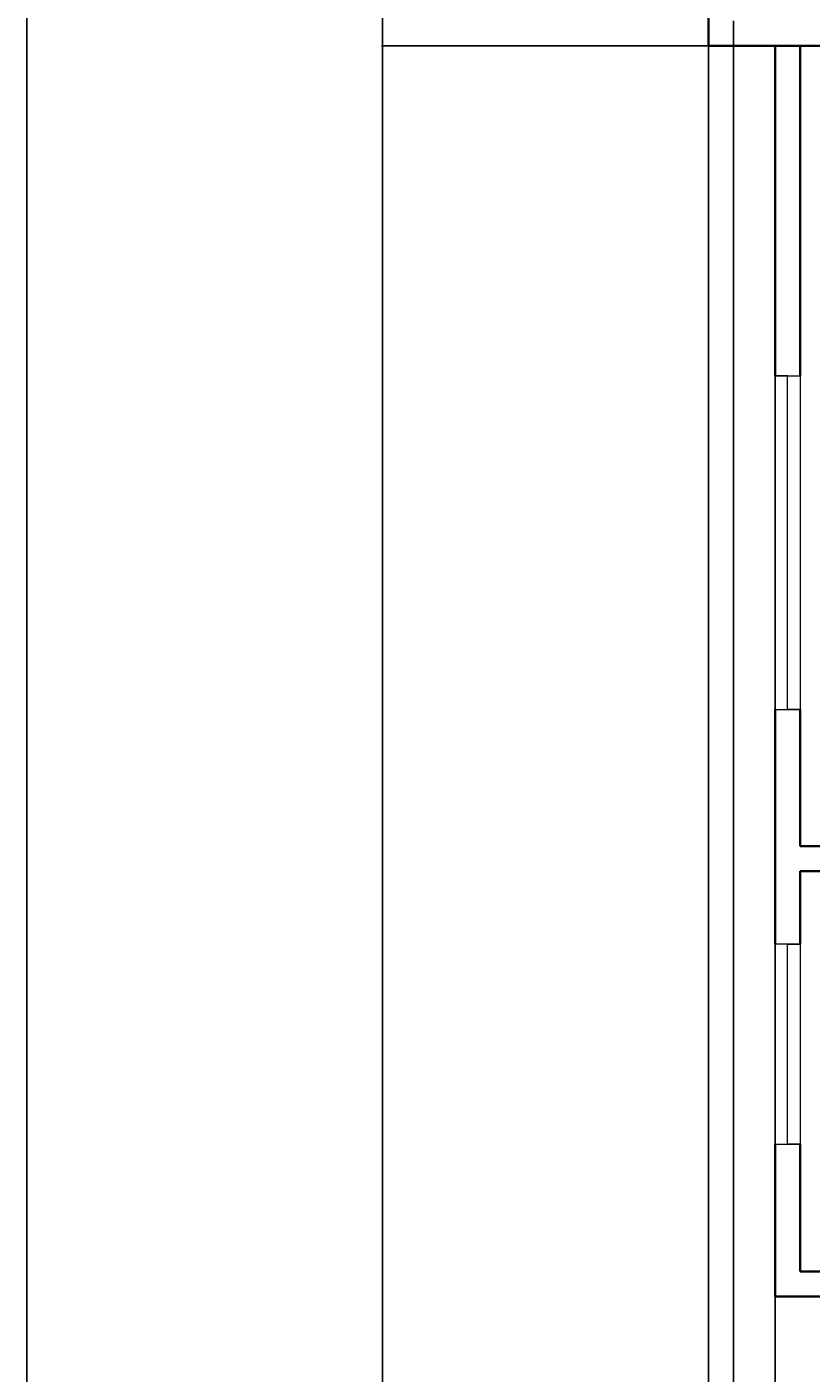
# Model space of a CAD drawing. Units: inches. Extents: x 2163 to 2982, y 1024 to 2288.
# Tile 2 of 22: x 2163 to 2304, y 1395 to 1637. Entities that reach past the tile are written whole.
import ezdxf

# ---------------------------------------------------------------- set-up
doc = ezdxf.new("R2010")
doc.units = ezdxf.units.IN
for name, color, linetype, lineweight in [('A-ANNO-DIMS', 2, 'Continuous', 18), ('A-ANNO-TTLB', 7, 'Continuous', 25), ('A-GLAZ', 161, 'Continuous', 18), ('A-WALL', 7, 'Continuous', 35)]:
    doc.layers.add(name, color=color, linetype=linetype, lineweight=lineweight)
doc.styles.get("Standard").update_dxf_attribs({"font": 'arial.ttf'})
doc.dimstyles.get("Standard").update_dxf_attribs({"dimtxt": 0.18, "dimasz": 0.18, "dimexe": 0.18, "dimexo": 0.0625, "dimgap": 0.09, "dimtad": 0, "dimtih": 1, "dimtoh": 1, "dimdec": 4, "dimzin": 0, "dimdsep": 46, "dimtxsty": 'Standard', "dimcen": 0.09, "dimadec": 0, "dimazin": 0, "dimtfac": 1, "dimtdec": 4, "dimtofl": 0, "dimtmove": 0, "dimatfit": 3, "dimfxl": 1, "dimtolj": 1, "dimtzin": 0, "dimarcsym": 0})

# ---------------------------------------------------------------- blocks, each defined once
blk = doc.blocks.new('WIN-60')
for p, q in [((2.25, 60), (0, 60)), ((0, 60), (4.5, 60)), ((0, 60), (0, 0)), ((2.25, 0), (2.25, 60)), ((4.5, 60), (4.5, 0)), ((0, 0), (4.5, 0)), ((4.5, 0), (2.25, 0))]:
    blk.add_line(p, q)
blk = doc.blocks.new('WIN-36-ALT')
for p, q in [((2.25, 36), (0, 36)), ((0, 36), (4.5, 36)), ((0, 36), (0, 0)), ((2.25, 0), (2.25, 36)), ((4.5, 36), (4.5, 0)), ((4.5, 0), (0, 0)), ((0, 0), (2.25, 0))]:
    blk.add_line(p, q)
blk = doc.blocks.new('*D30')
at = {"layer": 'A-ANNO-DIMS', "color": 0, "lineweight": -2, "transparency": 16777216}
for p, q in [((2285.34, 1633.71), (2285.34, 1023.79)), ((2297.34, 1633.71), (2297.34, 1023.79)), ((2285.52, 1023.97), (2291.13, 1023.97)), ((2297.16, 1023.97), (2291.55, 1023.97))]:
    blk.add_line(p, q, dxfattribs=at)
at = {"layer": 'A-ANNO-DIMS', "color": 0, "transparency": 16777216}
for points in [[(2285.52, 1024), (2285.52, 1023.94), (2285.34, 1023.97)], [(2297.16, 1024), (2297.16, 1023.94), (2297.34, 1023.97)]]:
    blk.add_solid(points, dxfattribs=at)
at = {"layer": 'Defpoints', "color": 0, "transparency": 16777216}
for p in [(2285.34, 1633.77), (2297.34, 1633.77), (2297.34, 1023.97)]:
    blk.add_point(p, dxfattribs=at)
at = {"layer": 'A-ANNO-DIMS', "color": 0, "transparency": 16777216, "insert": (2291.34, 1023.97), "char_height": 0.18, "attachment_point": 5}
blk.add_mtext('\\A1;12', dxfattribs=at)
blk = doc.blocks.new('*D33')
at = {"layer": 'A-ANNO-DIMS', "color": 0, "lineweight": -2, "transparency": 16777216}
for p, q in [((2285.28, 1633.77), (2226.51, 1633.77)), ((2226.69, 1633.59), (2226.69, 1388.7)), ((2226.69, 1143.45), (2226.69, 1388.34)), ((2297.28, 1143.27), (2226.51, 1143.27))]:
    blk.add_line(p, q, dxfattribs=at)
at = {"layer": 'A-ANNO-DIMS', "color": 0, "transparency": 16777216}
for points in [[(2226.66, 1633.59), (2226.72, 1633.59), (2226.69, 1633.77)], [(2226.66, 1143.45), (2226.72, 1143.45), (2226.69, 1143.27)]]:
    blk.add_solid(points, dxfattribs=at)
at = {"layer": 'Defpoints', "color": 0, "transparency": 16777216}
for p in [(2226.69, 1633.77), (2285.34, 1633.77), (2297.34, 1143.27)]:
    blk.add_point(p, dxfattribs=at)
at = {"layer": 'A-ANNO-DIMS', "color": 0, "transparency": 16777216, "insert": (2226.69, 1388.52), "char_height": 0.18, "attachment_point": 5}
blk.add_mtext('\\A1;490.5', dxfattribs=at)
blk = doc.blocks.new('*D34')
at = {"layer": 'A-ANNO-DIMS', "color": 0, "lineweight": -2, "transparency": 16777216}
for p, q in [((2285.28, 1738.77), (2226.51, 1738.77)), ((2226.69, 1738.59), (2226.69, 1686.45)), ((2226.69, 1633.95), (2226.69, 1686.09)), ((2285.28, 1633.77), (2226.51, 1633.77))]:
    blk.add_line(p, q, dxfattribs=at)
at = {"layer": 'A-ANNO-DIMS', "color": 0, "transparency": 16777216}
for points in [[(2226.66, 1738.59), (2226.72, 1738.59), (2226.69, 1738.77)], [(2226.66, 1633.95), (2226.72, 1633.95), (2226.69, 1633.77)]]:
    blk.add_solid(points, dxfattribs=at)
at = {"layer": 'Defpoints', "color": 0, "transparency": 16777216}
for p in [(2226.69, 1738.77), (2285.34, 1738.77), (2285.34, 1633.77)]:
    blk.add_point(p, dxfattribs=at)
at = {"layer": 'A-ANNO-DIMS', "color": 0, "transparency": 16777216, "insert": (2226.69, 1686.27), "char_height": 0.18, "attachment_point": 5}
blk.add_mtext('\\A1;105', dxfattribs=at)
blk = doc.blocks.new('*D36')
at = {"layer": 'A-ANNO-DIMS', "color": 0, "lineweight": -2, "transparency": 16777216}
for p, q in [((2289.84, 1638.21), (2289.84, 1023.79)), ((2329.44, 1638.21), (2329.44, 1023.79)), ((2290.02, 1023.97), (2309.18, 1023.97)), ((2329.26, 1023.97), (2310.11, 1023.97))]:
    blk.add_line(p, q, dxfattribs=at)
at = {"layer": 'A-ANNO-DIMS', "color": 0, "transparency": 16777216}
for points in [[(2290.02, 1024), (2290.02, 1023.94), (2289.84, 1023.97)], [(2329.26, 1024), (2329.26, 1023.94), (2329.44, 1023.97)]]:
    blk.add_solid(points, dxfattribs=at)
at = {"layer": 'Defpoints', "color": 0, "transparency": 16777216}
for p in [(2289.84, 1638.27), (2329.44, 1638.27), (2329.44, 1023.97)]:
    blk.add_point(p, dxfattribs=at)
at = {"layer": 'A-ANNO-DIMS', "color": 0, "transparency": 16777216, "insert": (2309.64, 1023.97), "char_height": 0.18, "attachment_point": 5}
blk.add_mtext('\\A1;39.605', dxfattribs=at)

msp = doc.modelspace()

# ---------------------------------------------------------------- linework, layer by layer
at = {"layer": 'A-ANNO-TTLB'}
msp.add_lwpolyline([(2162.6841, 2274.6054), (2982.469, 2274.6054), (2982.469, 1045.9691), (2162.6841, 1045.9691)], close=True, dxfattribs=at)
at = {"layer": 'A-WALL'}
for p, q in [((2285.3389, 1669.5085), (2285.3389, 1633.7688)), ((2285.3389, 1633.7688), (2301.8389, 1633.7688)), ((2297.3389, 1633.7688), (2297.3389, 1574.3679)), ((2301.8389, 1633.7688), (2445.8389, 1633.7688)), ((2301.8389, 1633.7688), (2301.8389, 1574.3679)), ((2297.3389, 1514.3679), (2297.3389, 1472.1506)), ((2301.8389, 1514.3679), (2301.8389, 1489.7688)), ((2301.8389, 1489.7688), (2445.8389, 1489.7688)), ((2301.8389, 1485.2688), (2445.8389, 1485.2688)), ((2301.8389, 1485.2688), (2301.8389, 1472.1506)), ((2297.3389, 1436.1506), (2297.3389, 1408.7688)), ((2301.8389, 1436.1506), (2301.8389, 1413.2688)), ((2301.8389, 1413.2688), (2425.632, 1413.2688)), ((2297.3389, 1408.7688), (2325.8389, 1408.7688))]:
    msp.add_line(p, q, dxfattribs=at)

# ---------------------------------------------------------------- block references
at = {"layer": 'A-GLAZ'}
msp.add_blockref('WIN-60', (2297.339, 1514.3679), dxfattribs=at)
at = {"layer": 'A-GLAZ', "extrusion": (0, 0, -1), "zscale": -1}
msp.add_blockref('WIN-36-ALT', (-2301.8388, 1436.1511), dxfattribs=at)

# ---------------------------------------------------------------- dimensions: what is measured, and where the dimension line sits
at = {"layer": 'A-ANNO-DIMS'}
for base, p1, p2, override, picture, middle in [((2226.6889, 1738.7688), (2285.3389, 1633.7688), (2285.3389, 1738.7688), {"dimdec": 0, "dimlfac": 1, "dimrnd": 0, "dimzin": 0, "dimdsep": 46, "dimlunit": 2}, '*D34', (2226.6889, 1686.2688)), ((2226.6889, 1633.7688), (2297.3389, 1143.2688), (2285.3389, 1633.7688), {"dimdec": 1, "dimlfac": 1, "dimrnd": 0, "dimzin": 0, "dimdsep": 46, "dimlunit": 2}, '*D33', (2226.6889, 1388.5188))]:
    dim = msp.add_linear_dim(base=base, p1=p1, p2=p2, angle=90, dimstyle='Standard', override=override, dxfattribs=at)
    dim.commit()
    dim.dimension.update_dxf_attribs({"geometry": picture, "text_midpoint": middle})
for base, p1, p2, override, picture, middle in [((2329.44344, 1023.97342), (2289.83891, 1638.26884), (2329.44344, 1638.26884), {"dimdec": 3, "dimlfac": 1, "dimrnd": 0, "dimzin": 0, "dimdsep": 46, "dimlunit": 2}, '*D36', (2309.64118, 1023.97342)), ((2297.3389, 1023.9734), (2285.3389, 1633.7688), (2297.3389, 1633.7688), {"dimdec": 0, "dimlfac": 1, "dimrnd": 0, "dimzin": 0, "dimdsep": 46, "dimlunit": 2}, '*D30', (2291.3389, 1023.9734))]:
    dim = msp.add_linear_dim(base=base, p1=p1, p2=p2, dimstyle='Standard', override=override, dxfattribs=at)
    dim.commit()
    dim.dimension.update_dxf_attribs({"geometry": picture, "text_midpoint": middle})

doc.saveas('drawing.dxf')
